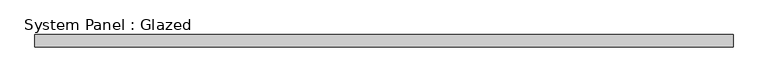
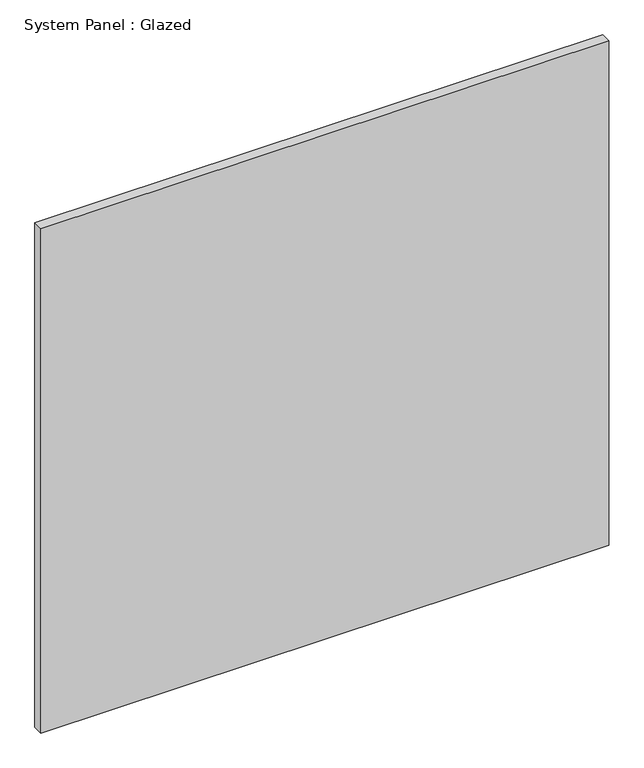
"""IFC4 building model written with IfcOpenShell, lengths in millimetres: plate geometry, System Panel : Glazed."""

from ifc_helpers import new_model, si_unit, origin, origin_with_axes, place, context, project, spatial, polyline, outline, extrude, source, transform, mapped, element, save


def system_panel_glazed_7e3392a4(model_context):
    return source(origin(), model_context, "Body", "SweptSolid", [
        extrude(outline(polyline([(708.7455726, 24.5), (-708.7455726, 24.5), (-708.7455726, 49.5), (708.7455726, 49.5), (708.7455726, 24.5)])), origin_with_axes(), (0.0, 0.0, 1.0), 1330.8429687),
    ])


if __name__ == "__main__":
    model = new_model("IFC4")
    model_context = context("Model", 3, world=origin())
    ifc_project = project(units=[si_unit("LENGTHUNIT", "METRE", prefix="MILLI")], contexts=[model_context])
    site = spatial("IfcSite", under=ifc_project)
    building = spatial("IfcBuilding", under=site)
    placement = place(None, origin())
    system_panel_glazed_shape = system_panel_glazed_7e3392a4(model_context)
    element("IfcPlate", 1, ObjectType="System Panel : Glazed", at=placement, inside=building, context=model_context, shape_type="MappedRepresentation", body=[
        mapped(system_panel_glazed_shape, transform((0.0, 0.0, 0.0), x_axis=(1.0, 0.0, 0.0), y_axis=(0.0, 1.0, 0.0), z_axis=(0.0, 0.0, 1.0))),
    ])
    save(model, "model.ifc")

# Revit data of these elements
# Type "System Panel : Glazed"
#   Keynote = "H11"
#   Construction Type Id = "GSP4R"
#   Analytic Construction = "1/8 in Pilkington single glazing"
#   Visual Light Transmittance = 0.9
#   Solar Heat Gain Coefficient = 0.86
#   Heat Transfer Coefficient (U) = 6.7069 W/(m²·K)
#   Define Thermal Properties by = 1
# Element 1 (IfcPlate, "System Panel : Glazed")
#   Materials on its faces: "Glass"
# Materials
#   "Glass": class "Glass", colour RGB 0 128 192, transparency 0.9, Description = "Soda Lime Glass", Cost = 0
